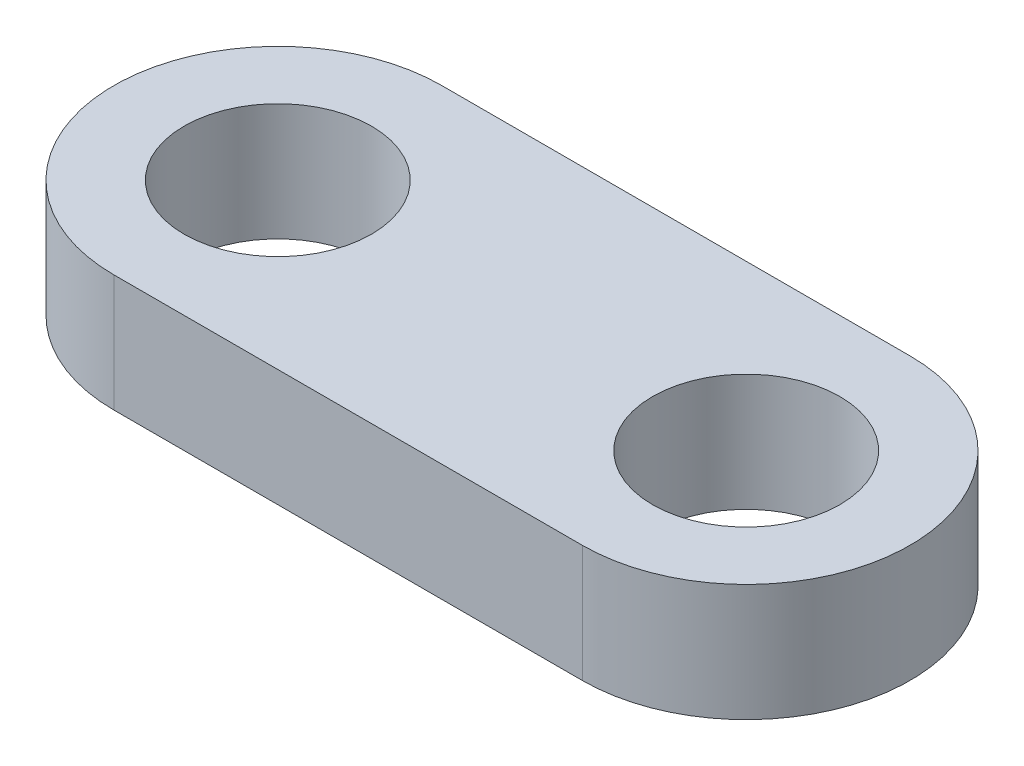
from build123d import *

# Parameters (mm, degrees)
LINK_PLATE_DEPTH         = 2.5
HOLE_SKETCH_R            = 4
THROUGH_HOLES_2X_8_DEPTH = 2.5


with BuildPart() as part:
    # Link Profile Sketch → Link Plate (new, symmetric)
    with BuildSketch(Plane(origin=(0, 0, 0), x_dir=(1, 0, 0), z_dir=(0, 1, 0))):
        with BuildLine():
            Line((-10, 7), (10, 7))
            ThreePointArc((10, 7), (17, 0), (10, -7))
            Line((10, -7), (-10, -7))
            ThreePointArc((-10, -7), (-17, 0), (-10, 7))
        make_face()
    extrude(amount=LINK_PLATE_DEPTH, both=True)

    # Hole Sketch → Through Holes 2xØ8 (cut, symmetric)
    with BuildSketch(Plane(origin=(0, 0, 0), x_dir=(1, 0, 0), z_dir=(0, 1, 0))):
        with Locations(Location((10, 0, 0), (0, 0, 270))):
            Circle(HOLE_SKETCH_R)
        with Locations(Location((-10, 0, 0), (0, 0, 270))):
            Circle(HOLE_SKETCH_R)
    extrude(amount=THROUGH_HOLES_2X_8_DEPTH, both=True, mode=Mode.SUBTRACT)


solid = part.part
